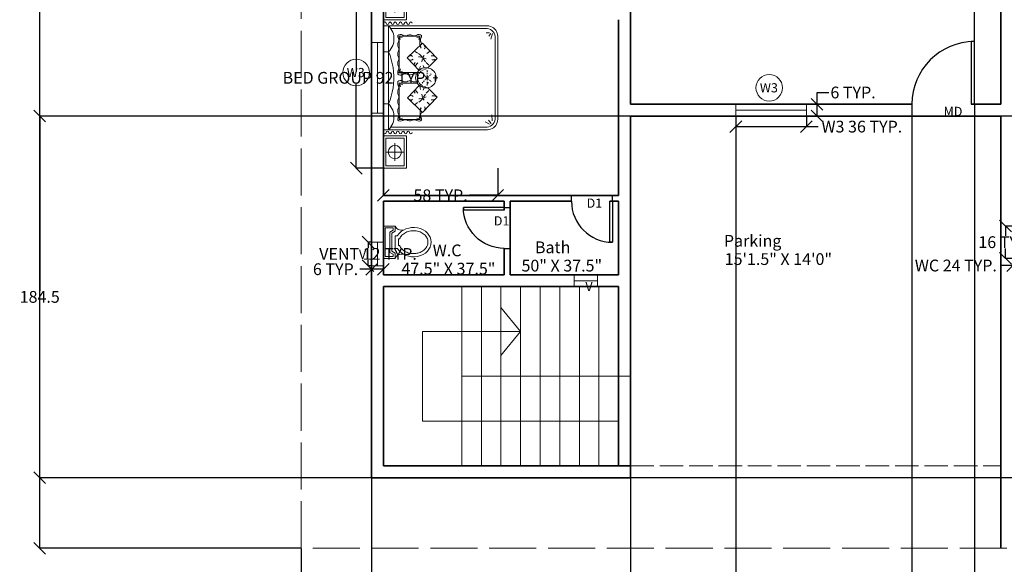
# Model space of a CAD drawing. Units: inches. Extents: x -1198 to -69, y -512 to 437.
# Tile 2 of 50: x -1198 to -696, y -273 to 5. Entities that reach past the tile are written whole.
import ezdxf

# ---------------------------------------------------------------- set-up
doc = ezdxf.new("R2010")
doc.units = ezdxf.units.IN
doc.header["$MEASUREMENT"] = 0
doc.linetypes.add('ACAD_ISO02W100', pattern=[15, 12, -3])
for name, color, linetype, lineweight in [('A-ANNO-DIMS', 2, 'Continuous', 18), ('A-ANNO-SYMB', 7, 'Continuous', 18), ('A-AREA-IDEN', 7, 'Continuous', 18), ('A-FLOR-FIXT', 60, 'Continuous', 18), ('A-FLOR-OPEN', 7, 'ACAD_ISO02W100', 18), ('A-FLOR-STRS', 7, 'Continuous', 18), ('A-FURN', 60, 'Continuous', 18), ('A-WALL', 7, 'Continuous', 35), ('C-PROP', 141, 'ACAD_ISO02W100', 18), ('Doors', 140, 'Continuous', 25), ('ds_furniture_Pen_No__7', 7, 'Continuous', 18), ('windows', 160, 'Continuous', 18)]:
    doc.layers.add(name, color=color, linetype=linetype, lineweight=lineweight)
doc.styles.get("Standard").update_dxf_attribs({"font": 'arial.ttf'})
doc.dimstyles.get("Standard").update_dxf_attribs({"dimtxt": 6, "dimasz": 6, "dimexe": 0.18, "dimexo": 0.0625, "dimgap": 0.09, "dimtad": 0, "dimtih": 1, "dimtoh": 1, "dimdec": 0, "dimzin": 0, "dimdsep": 46, "dimlunit": 4, "dimtxsty": 'Standard', "dimblk": 'OBLIQUE', "dimcen": 0.09, "dimadec": 0, "dimazin": 0, "dimtfac": 1, "dimtdec": 0, "dimtofl": 0, "dimtmove": 0, "dimatfit": 3, "dimfxl": 1, "dimtolj": 1, "dimtzin": 0, "dimarcsym": 0})

# ---------------------------------------------------------------- blocks, each defined once
blk = doc.blocks.new('*U5')
for p, q in [((0, 0), (0, -6)), ((-32, 0), (-32, -6))]:
    blk.add_line(p, q)
blk.add_lwpolyline([(0, 0), (0, 32), (-1.75, 32), (-1.75, 0)], close=True)
blk.add_arc((0, 0), 32, 90, 180)
blk = doc.blocks.new('new')
at = {"layer": 'ds_furniture_Pen_No__7'}
for p, q in [((-1180, 2274), (-1838, 2274)), ((-1838, 2274), (-1838, 1804)), ((-1227, 2227), (-1791, 2227)), ((-1791, 2227), (-1791, 1851)), ((-1509, 2220), (-1509, 1858)), ((-1227, 1851), (-1227, 2227)), ((-1180, 1804), (-1180, 2274)), ((-1058, 159), (-1058, 2274)), ((-1058, 2274), (1058, 2274)), ((-1058, 2274), (1058, 2274)), ((-1058, 159), (-1058, 2274)), ((-529, 2274), (-529, 2169)), ((529, 2274), (529, 2169)), ((1058, 2274), (1058, 159)), ((1058, 2274), (1058, 159)), ((1180, 1804), (1180, 2274)), ((1180, 2274), (1838, 2274)), ((1227, 1851), (1227, 2227)), ((1227, 2227), (1791, 2227)), ((1509, 2220), (1509, 1858)), ((1791, 2227), (1791, 1851)), ((1838, 2274), (1838, 1804)), ((-1690, 2039), (-1328, 2039)), ((1058, 2169), (-1058, 2169)), ((-1058, 2169), (-1028, 2143)), ((-1028, 2143), (-996, 2120)), ((-1005, 165), (-1005, 2124)), ((-996, 2120), (-963, 2101)), ((-963, 2101), (-927, 2084)), ((-927, 2084), (-891, 2071)), ((-891, 2071), (-851, 2063)), ((-851, 2063), (-812, 2059)), ((-812, 2059), (-772, 2059)), ((-772, 2059), (-734, 2063)), ((-734, 2063), (-696, 2071)), ((-696, 2071), (-658, 2084)), ((-658, 2084), (-622, 2101)), ((-622, 2101), (-588, 2120)), ((-588, 2120), (-556, 2143)), ((-556, 2143), (-529, 2169)), ((-529, 2169), (-451, 2139)), ((-451, 2139), (-370, 2114)), ((-370, 2114), (-290, 2092)), ((-290, 2092), (-207, 2075)), ((-207, 2075), (-125, 2065)), ((-125, 2065), (-42, 2061)), ((-42, 2061), (42, 2061)), ((42, 2061), (125, 2065)), ((125, 2065), (207, 2075)), ((207, 2075), (290, 2092)), ((290, 2092), (370, 2114)), ((370, 2114), (451, 2139)), ((451, 2139), (529, 2169)), ((529, 2169), (556, 2143)), ((556, 2143), (588, 2120)), ((588, 2120), (622, 2101)), ((622, 2101), (658, 2084)), ((658, 2084), (696, 2071)), ((696, 2071), (734, 2063)), ((734, 2063), (772, 2059)), ((772, 2059), (812, 2059)), ((812, 2059), (851, 2063)), ((851, 2063), (891, 2071)), ((891, 2071), (927, 2084)), ((927, 2084), (963, 2101)), ((963, 2101), (996, 2120)), ((996, 2120), (1028, 2143)), ((1005, 2124), (1005, 165)), ((1028, 2143), (1058, 2169)), ((1690, 2039), (1328, 2039)), ((-1838, 1804), (-1180, 1804)), ((-1791, 1851), (-1227, 1851)), ((-880, 1932), (-874, 1959)), ((-878, 1904), (-880, 1932)), ((-870, 1879), (-878, 1904)), ((-874, 1959), (-861, 1982)), ((-857, 1855), (-870, 1879)), ((-861, 1982), (-836, 1982)), ((-857, 1798), (-857, 1855)), ((-846, 1528), (-846, 1951)), ((-846, 1951), (-108, 1951)), ((-836, 1982), (-810, 1974)), ((-831, 1930), (-821, 1887)), ((-825, 1944), (-779, 1930)), ((-810, 1974), (-787, 1961)), ((-787, 1961), (-751, 1961)), ((-751, 1961), (-726, 1974)), ((-726, 1974), (-700, 1980)), ((-700, 1980), (-675, 1982)), ((-675, 1982), (-647, 1980)), ((-647, 1980), (-622, 1974)), ((-622, 1974), (-597, 1961)), ((-597, 1961), (-561, 1961)), ((-561, 1961), (-535, 1974)), ((-535, 1974), (-510, 1980)), ((-510, 1980), (-484, 1982)), ((-484, 1982), (-457, 1980)), ((-457, 1980), (-432, 1974)), ((-432, 1974), (-408, 1961)), ((-408, 1961), (-370, 1961)), ((-370, 1961), (-347, 1974)), ((-347, 1974), (-322, 1980)), ((-322, 1980), (-294, 1982)), ((-294, 1982), (-267, 1980)), ((-267, 1980), (-241, 1974)), ((-241, 1974), (-218, 1961)), ((-218, 1961), (-180, 1961)), ((-133, 1940), (-182, 1923)), ((-180, 1961), (-157, 1974)), ((-157, 1974), (-133, 1982)), ((-129, 1923), (-140, 1881)), ((-133, 1982), (-106, 1982)), ((-108, 1951), (-108, 1591)), ((-106, 1982), (-74, 1982)), ((-66, 1879), (-80, 1855)), ((-80, 1855), (-80, 1798)), ((-74, 1982), (-63, 1959)), ((-57, 1904), (-66, 1879)), ((-63, 1959), (-57, 1932)), ((-57, 1932), (-57, 1904)), ((63, 1959), (57, 1932)), ((57, 1932), (57, 1904)), ((57, 1904), (66, 1879)), ((74, 1982), (63, 1959)), ((66, 1879), (80, 1855)), ((106, 1982), (74, 1982)), ((80, 1855), (80, 1798)), ((133, 1982), (106, 1982)), ((844, 1953), (106, 1953)), ((106, 1953), (106, 1593)), ((127, 1925), (138, 1883)), ((131, 1942), (180, 1925)), ((157, 1974), (133, 1982)), ((180, 1961), (157, 1974)), ((218, 1961), (180, 1961)), ((241, 1974), (218, 1961)), ((267, 1980), (241, 1974)), ((294, 1982), (267, 1980)), ((322, 1980), (294, 1982)), ((347, 1974), (322, 1980)), ((370, 1961), (347, 1974)), ((408, 1961), (370, 1961)), ((432, 1974), (408, 1961)), ((457, 1980), (432, 1974)), ((484, 1982), (457, 1980)), ((510, 1980), (484, 1982)), ((535, 1974), (510, 1980)), ((561, 1961), (535, 1974)), ((597, 1961), (561, 1961)), ((622, 1974), (597, 1961)), ((647, 1980), (622, 1974)), ((675, 1982), (647, 1980)), ((700, 1980), (675, 1982)), ((726, 1974), (700, 1980)), ((751, 1961), (726, 1974)), ((787, 1961), (751, 1961)), ((823, 1946), (776, 1932)), ((810, 1974), (787, 1961)), ((836, 1982), (810, 1974)), ((829, 1932), (819, 1889)), ((861, 1982), (836, 1982)), ((844, 1530), (844, 1953)), ((857, 1855), (870, 1879)), ((857, 1798), (857, 1855)), ((874, 1959), (861, 1982)), ((870, 1879), (878, 1904)), ((880, 1932), (874, 1959)), ((878, 1904), (880, 1932)), ((1838, 1804), (1180, 1804)), ((1791, 1851), (1227, 1851)), ((-876, 1748), (-870, 1775)), ((-876, 1722), (-876, 1748)), ((-870, 1695), (-876, 1722)), ((-870, 1775), (-857, 1798)), ((-857, 1671), (-870, 1695)), ((-870, 1602), (-857, 1625)), ((-857, 1625), (-857, 1671)), ((-705, 1475), (-408, 1786)), ((-540, 1627), (-504, 1580)), ((-440, 1743), (-461, 1707)), ((-461, 1707), (-436, 1680)), ((-408, 1786), (-154, 1544)), ((-362, 1697), (-383, 1669)), ((-366, 1750), (-362, 1697)), ((-277, 1648), (-313, 1627)), ((-245, 1627), (-309, 1574)), ((-91, 1595), (-61, 1608)), ((-80, 1798), (-66, 1775)), ((-66, 1695), (-80, 1671)), ((-80, 1671), (-80, 1608)), ((-66, 1775), (-59, 1748)), ((-59, 1722), (-66, 1695)), ((-61, 1608), (-32, 1614)), ((-59, 1748), (-59, 1722)), ((-32, 1614), (0, 1619)), ((0, 1619), (32, 1614)), ((32, 1614), (61, 1608)), ((66, 1775), (59, 1748)), ((59, 1748), (59, 1722)), ((59, 1722), (66, 1695)), ((61, 1608), (91, 1595)), ((80, 1798), (66, 1775)), ((66, 1695), (80, 1671)), ((80, 1671), (80, 1608)), ((406, 1788), (152, 1547)), ((243, 1629), (307, 1576)), ((275, 1650), (311, 1629)), ((364, 1752), (360, 1699)), ((360, 1699), (381, 1671)), ((702, 1477), (406, 1788)), ((459, 1709), (434, 1682)), ((438, 1745), (459, 1709)), ((537, 1629), (501, 1583)), ((870, 1775), (857, 1798)), ((857, 1671), (870, 1695)), ((857, 1625), (857, 1671)), ((870, 1602), (857, 1625)), ((876, 1748), (870, 1775)), ((870, 1695), (876, 1722)), ((876, 1722), (876, 1748)), ((-880, 1549), (-878, 1576)), ((-874, 1521), (-880, 1549)), ((-878, 1576), (-870, 1602)), ((-861, 1498), (-874, 1521)), ((-836, 1498), (-861, 1498)), ((-652, 1528), (-846, 1528)), ((-810, 1506), (-836, 1498)), ((-831, 1549), (-821, 1591)), ((-825, 1534), (-779, 1549)), ((-787, 1519), (-810, 1506)), ((-772, 1517), (-789, 1517)), ((-751, 1519), (-787, 1519)), ((-762, 1517), (-772, 1517)), ((-751, 1517), (-762, 1517)), ((-726, 1506), (-751, 1519)), ((-700, 1500), (-726, 1506)), ((-394, 1178), (-705, 1475)), ((-683, 1498), (-700, 1500)), ((-656, 1517), (-635, 1517)), ((-656, 1439), (-620, 1422)), ((-635, 1517), (-614, 1506)), ((-614, 1506), (-630, 1517)), ((-630, 1517), (-603, 1513)), ((-620, 1422), (-599, 1432)), ((-599, 1432), (-588, 1439)), ((-472, 1523), (-493, 1555)), ((-425, 1481), (-472, 1523)), ((-457, 1443), (-419, 1470)), ((-429, 1538), (-429, 1555)), ((-415, 1481), (-429, 1538)), ((-404, 1443), (-415, 1481)), ((-398, 1475), (-330, 1492)), ((-398, 1439), (-387, 1401)), ((-394, 1460), (-330, 1418)), ((-218, 1449), (-250, 1464)), ((-214, 1528), (-239, 1517)), ((-218, 1449), (-203, 1449)), ((-176, 1528), (-214, 1528)), ((-205, 1418), (-201, 1449)), ((-205, 1386), (-205, 1418)), ((-201, 1449), (-193, 1479)), ((-197, 1401), (-180, 1439)), ((-193, 1479), (-180, 1508)), ((-182, 1555), (-154, 1544)), ((-180, 1508), (-163, 1534)), ((-176, 1528), (-171, 1523)), ((-169, 1479), (-176, 1458)), ((-169, 1479), (-159, 1489)), ((-163, 1534), (-142, 1557)), ((-116, 1538), (-148, 1500)), ((-148, 1528), (-144, 1521)), ((-142, 1557), (-118, 1578)), ((-118, 1578), (-91, 1595)), ((-116, 1538), (-95, 1549)), ((-91, 1468), (-106, 1485)), ((-59, 1443), (-80, 1458)), ((-42, 1574), (-74, 1559)), ((-38, 1428), (-49, 1428)), ((-32, 1580), (-2, 1580)), ((-6, 1396), (-32, 1418)), ((19, 1580), (-11, 1580)), ((-6, 1585), (-6, 1570)), ((-6, 1585), (-6, 1570)), ((4, 1396), (30, 1418)), ((30, 1574), (61, 1559)), ((36, 1428), (47, 1428)), ((57, 1443), (78, 1458)), ((104, 1538), (83, 1549)), ((89, 1468), (104, 1485)), ((91, 1595), (118, 1578)), ((112, 1528), (138, 1502)), ((118, 1578), (142, 1557)), ((142, 1557), (163, 1534)), ((157, 1479), (146, 1489)), ((180, 1557), (152, 1547)), ((157, 1479), (163, 1458)), ((163, 1534), (180, 1508)), ((184, 1401), (167, 1439)), ((173, 1530), (169, 1525)), ((173, 1530), (212, 1530)), ((180, 1508), (193, 1479)), ((193, 1479), (201, 1449)), ((216, 1451), (201, 1451)), ((201, 1449), (205, 1418)), ((205, 1418), (205, 1386)), ((212, 1530), (237, 1519)), ((216, 1451), (248, 1466)), ((258, 1350), (311, 1403)), ((396, 1477), (328, 1494)), ((391, 1462), (328, 1420)), ((396, 1441), (385, 1403)), ((391, 1181), (702, 1477)), ((402, 1445), (413, 1483)), ((413, 1483), (427, 1540)), ((455, 1445), (417, 1473)), ((423, 1483), (470, 1525)), ((427, 1540), (427, 1557)), ((470, 1525), (491, 1557)), ((597, 1434), (586, 1441)), ((618, 1424), (597, 1434)), ((628, 1519), (601, 1515)), ((633, 1519), (611, 1508)), ((611, 1508), (628, 1519)), ((654, 1441), (618, 1424)), ((654, 1519), (633, 1519)), ((650, 1530), (844, 1530)), ((683, 1498), (700, 1500)), ((700, 1500), (726, 1506)), ((726, 1506), (751, 1519)), ((749, 1519), (760, 1519)), ((751, 1519), (787, 1519)), ((760, 1519), (770, 1519)), ((770, 1519), (787, 1519)), ((823, 1536), (776, 1551)), ((787, 1519), (810, 1506)), ((810, 1506), (836, 1498)), ((829, 1551), (819, 1593)), ((836, 1498), (861, 1498)), ((861, 1498), (874, 1521)), ((878, 1576), (870, 1602)), ((874, 1521), (880, 1549)), ((880, 1549), (878, 1576)), ((-540, 1333), (-493, 1386)), ((-451, 1274), (-446, 1301)), ((-451, 1252), (-451, 1274)), ((-436, 1227), (-451, 1252)), ((-394, 1178), (-207, 1369)), ((-383, 1217), (-366, 1238)), ((-366, 1280), (-372, 1280)), ((-366, 1238), (-366, 1280)), ((-260, 1348), (-313, 1401)), ((-199, 1356), (-205, 1386)), ((-188, 1324), (-199, 1356)), ((-176, 1297), (-188, 1324)), ((-157, 1272), (-176, 1297)), ((-123, 1386), (-159, 1386)), ((-133, 1248), (-157, 1272)), ((-110, 1229), (-133, 1248)), ((-80, 1214), (-110, 1229)), ((-80, 1386), (-106, 1386)), ((-74, 1312), (-80, 1301)), ((-51, 1204), (-80, 1214)), ((53, 1221), (-72, 1221)), ((-59, 1386), (-63, 1386)), ((-49, 1333), (-63, 1316)), ((-21, 1197), (-51, 1204)), ((-17, 1375), (-49, 1386)), ((-38, 1343), (-38, 1343)), ((-6, 1369), (-32, 1354)), ((-17, 1386), (-17, 1396)), ((-17, 1396), (-6, 1396)), ((-17, 1375), (-17, 1386)), ((-6, 1369), (-17, 1375)), ((-6, 1396), (-2, 1398)), ((-6, 1369), (-2, 1369)), ((4, 1396), (-2, 1398)), ((4, 1369), (-2, 1369)), ((0, 1164), (0, 1263)), ((15, 1396), (4, 1396)), ((4, 1369), (15, 1375)), ((4, 1369), (30, 1354)), ((15, 1386), (15, 1396)), ((15, 1375), (15, 1386)), ((15, 1375), (47, 1386)), ((51, 1204), (21, 1197)), ((36, 1343), (36, 1343)), ((47, 1333), (61, 1316)), ((80, 1214), (51, 1204)), ((57, 1386), (61, 1386)), ((72, 1312), (78, 1301)), ((78, 1386), (104, 1386)), ((110, 1229), (80, 1214)), ((133, 1248), (110, 1229)), ((121, 1386), (157, 1386)), ((157, 1272), (133, 1248)), ((176, 1297), (157, 1272)), ((188, 1324), (176, 1297)), ((199, 1356), (188, 1324)), ((205, 1386), (199, 1356)), ((391, 1181), (205, 1371)), ((364, 1240), (364, 1282)), ((364, 1282), (370, 1282)), ((381, 1219), (364, 1240)), ((434, 1229), (449, 1255)), ((449, 1276), (444, 1303)), ((449, 1255), (449, 1276)), ((537, 1335), (491, 1388)), ((0, 1197), (-21, 1197)), ((21, 1197), (0, 1197)), ((-941, 116), (-895, 205)), ((-1054, 127), (-1058, 159)), ((-1054, 127), (-1058, 159)), ((-1045, 95), (-1054, 127)), ((-1045, 95), (-1054, 127)), ((-1032, 63), (-1045, 95)), ((-1032, 63), (-1045, 95)), ((-1016, 36), (-1032, 63)), ((-1016, 36), (-1032, 63)), ((-994, 11), (-1016, 36)), ((-994, 11), (-1016, 36)), ((-996, 129), (-1005, 165)), ((-984, 97), (-996, 129)), ((-969, -11), (-994, 11)), ((-969, -11), (-994, 11)), ((-963, 68), (-984, 97)), ((-937, 42), (-963, 68)), ((-908, 21), (-937, 42)), ((-931, 85), (-863, 138)), ((-876, 8), (-908, 21)), ((-840, 0), (-876, 8)), ((-874, 63), (-751, 70)), ((840, 0), (-840, 0)), ((903, 53), (787, 91)), ((876, 8), (840, 0)), ((903, 91), (844, 127)), ((908, 21), (876, 8)), ((937, 42), (908, 21)), ((914, 116), (914, 184)), ((963, 68), (937, 42)), ((984, 97), (963, 68)), ((994, 11), (969, -11)), ((994, 11), (969, -11)), ((996, 129), (984, 97)), ((1016, 36), (994, 11)), ((1016, 36), (994, 11)), ((1005, 165), (996, 129)), ((1032, 63), (1016, 36)), ((1032, 63), (1016, 36)), ((1045, 95), (1032, 63)), ((1045, 95), (1032, 63)), ((1054, 127), (1045, 95)), ((1054, 127), (1045, 95)), ((1058, 159), (1054, 127)), ((1058, 159), (1054, 127)), ((-941, -28), (-969, -11)), ((-941, -28), (-969, -11)), ((-910, -40), (-941, -28)), ((-910, -40), (-941, -28)), ((-878, -49), (-910, -40)), ((-878, -49), (-910, -40)), ((-846, -53), (-878, -49)), ((-846, -53), (-878, -49)), ((846, -53), (-846, -53)), ((846, -53), (-846, -53)), ((878, -49), (846, -53)), ((878, -49), (846, -53)), ((910, -40), (878, -49)), ((910, -40), (878, -49)), ((941, -28), (910, -40)), ((941, -28), (910, -40)), ((969, -11), (941, -28)), ((969, -11), (941, -28))]:
    blk.add_line(p, q, dxfattribs=at)
for centre in [(-1509, 2039), (1509, 2039)]:
    blk.add_circle(centre, 134, dxfattribs=at)
for centre, start, end in [((-1113, 2243), 90, 270), ((-1113, 2191), 270, 90), ((1109, 2191), 90, 270), ((1109, 2243), 270, 90), ((-1113, 2138), 90, 270), ((-1113, 2032), 90, 270), ((-1113, 2085), 270, 90), ((-1113, 2085), 270, 90), ((-1113, 1979), 270, 90), ((1109, 2085), 90, 270), ((1109, 2085), 90, 270), ((1109, 1979), 90, 270), ((1109, 2138), 270, 90), ((1109, 2032), 270, 90), ((-1113, 1926), 90, 270), ((-1113, 1820), 90, 270), ((-1113, 1873), 270, 90), ((1109, 1873), 90, 270), ((1109, 1926), 270, 90), ((1109, 1820), 270, 90), ((-1113, 1715), 90, 270), ((-1113, 1767), 270, 90), ((1109, 1767), 90, 270), ((1109, 1715), 270, 90)]:
    blk.add_arc(centre, 26.4, start, end, dxfattribs=at)
blk = doc.blocks.new('A$C7C8779AE')
for p, q in [((0, 0.74), (0, 0.56)), ((0.5, 0.74), (0, 0.74)), ((0.47, 0.71), (0.03, 0.71)), ((0.03, 0.71), (0.03, 0.59)), ((0.093, 0.64), (0.063, 0.59)), ((0.11, 0.61), (0.08, 0.56)), ((0.093, 0.64), (0.407, 0.64)), ((0.11, 0.61), (0.39, 0.61)), ((0.42, 0.56), (0.39, 0.61)), ((0.437, 0.59), (0.407, 0.64)), ((0.47, 0.59), (0.47, 0.71)), ((0.5, 0.56), (0.5, 0.74)), ((0, 0.56), (0.08, 0.56)), ((0.03, 0.59), (0.063, 0.59)), ((0.15, 0.557), (0.15, 0.52)), ((0.15, 0.557), (0.351, 0.557)), ((0.2, 0.507), (0.2, 0.488)), ((0.2, 0.507), (0.301, 0.507)), ((0.301, 0.507), (0.301, 0.488)), ((0.351, 0.557), (0.351, 0.52)), ((0.42, 0.56), (0.5, 0.56)), ((0.437, 0.59), (0.47, 0.59))]:
    blk.add_line(p, q)
for centre, start, end in [((-0.039, 0.461), 344.642, 68.7339), ((0.539, 0.461), 111.2661, 195.358)]:
    blk.add_arc(centre, 0.106, start, end)
blk.add_ellipse((0.251, 0.274), major_axis=(0, 0.274), ratio=0.828948, start_param=0.459479, end_param=5.823706)
blk.add_open_spline([(0.2, 0.488), (0.17, 0.474), (0.164, 0.47), (0.151, 0.46), (0.144, 0.454), (0.13, 0.439), (0.123, 0.431), (0.111, 0.413), (0.106, 0.404), (0.096, 0.384), (0.091, 0.373), (0.084, 0.352), (0.081, 0.34), (0.076, 0.317), (0.075, 0.305), (0.073, 0.282), (0.073, 0.27), (0.074, 0.246), (0.076, 0.234), (0.08, 0.211), (0.083, 0.2), (0.09, 0.178), (0.095, 0.167), (0.104, 0.147), (0.11, 0.138), (0.122, 0.12), (0.128, 0.112), (0.142, 0.097), (0.149, 0.09), (0.165, 0.078), (0.173, 0.073), (0.189, 0.064), (0.197, 0.06), (0.214, 0.055), (0.222, 0.053), (0.239, 0.05), (0.248, 0.05), (0.266, 0.051), (0.276, 0.052), (0.296, 0.057), (0.306, 0.061), (0.325, 0.071), (0.335, 0.077), (0.353, 0.091), (0.361, 0.099), (0.377, 0.117), (0.384, 0.127), (0.398, 0.149), (0.404, 0.161), (0.414, 0.185), (0.418, 0.198), (0.424, 0.225), (0.426, 0.239), (0.428, 0.267), (0.428, 0.281), (0.426, 0.309), (0.424, 0.323), (0.418, 0.349), (0.414, 0.363), (0.404, 0.387), (0.398, 0.399), (0.385, 0.421), (0.378, 0.431), (0.362, 0.449), (0.353, 0.458), (0.338, 0.469), (0.332, 0.474), (0.301, 0.488)], degree=3, knots=[0.459479, 0.459479, 0.459479, 0.459479, 0.567422, 0.567422, 0.720865, 0.720865, 0.874307, 0.874307, 1.02775, 1.02775, 1.181192, 1.181192, 1.334635, 1.334635, 1.488077, 1.488077, 1.64152, 1.64152, 1.794963, 1.794963, 1.948405, 1.948405, 2.101848, 2.101848, 2.25529, 2.25529, 2.408733, 2.408733, 2.562175, 2.562175, 2.715618, 2.715618, 2.86906, 2.86906, 3.022503, 3.022503, 3.175946, 3.175946, 3.356457, 3.356457, 3.536968, 3.536968, 3.717479, 3.717479, 3.89799, 3.89799, 4.078501, 4.078501, 4.259012, 4.259012, 4.439523, 4.439523, 4.620035, 4.620035, 4.800546, 4.800546, 4.981057, 4.981057, 5.161568, 5.161568, 5.342079, 5.342079, 5.52259, 5.52259, 5.703101, 5.703101, 5.823706, 5.823706, 5.823706, 5.823706])
blk = doc.blocks.new('A')
at = {"xscale": 1000, "yscale": 1000, "zscale": 1000}
blk.add_blockref('A$C7C8779AE', (-251, 0), dxfattribs=at)
blk = doc.blocks.new('WIN-W3-36')
at = {"ltscale": 10}
for p, q in [((0, 6), (0, 0)), ((36, 6), (36, 0)), ((0, 3), (36, 3))]:
    blk.add_line(p, q, dxfattribs=at)
blk = doc.blocks.new('VENT-12')
at = {"ltscale": 10}
for p, q in [((0, 6), (0, 0)), ((12, 6), (12, 0)), ((0, 3), (12, 3))]:
    blk.add_line(p, q, dxfattribs=at)
blk = doc.blocks.new('DOOR-D1-JAMB3')
for p, q in [((0, 0), (0, -3)), ((20.87, 0), (20.87, -3))]:
    blk.add_line(p, q)
blk.add_lwpolyline([(0, 0), (0, 20.87), (1.3, 20.87), (1.3, 0)], close=True)
blk.add_arc((0, 0), 20.87, 0, 90)
blk = doc.blocks.new('STAIR-RETURN')
at = {"ltscale": 10}
for p, q in [((20, 91.5), (20, 0)), ((30, 91.5), (30, 0)), ((40, 91.5), (40, 0)), ((50, 91.5), (50, 0)), ((60, 91.5), (60, 0)), ((70, 91.5), (70, 0)), ((80, 91.5), (80, 0)), ((90, 91.5), (90, 0)), ((50, 68.62), (40, 80.86)), ((0, 22.87), (0, 68.62)), ((0, 68.62), (50, 68.62)), ((50, 68.62), (40, 56.39)), ((20, 45.75), (106, 45.75)), ((100, 22.87), (0, 22.87))]:
    blk.add_line(p, q, dxfattribs=at)
blk = doc.blocks.new('TAG-W3')
at = {"ltscale": 10}
blk.add_circle((0, 0), 6.77, dxfattribs=at)
blk.add_text('W3', height=4.7, dxfattribs=at).set_placement((-4.79, -2.36))
blk = doc.blocks.new('_Oblique')
at = {"color": 0, "linetype": 'ByBlock', "lineweight": -2}
blk.add_line((-0.5, -0.5), (0.5, 0.5), dxfattribs=at)
blk = doc.blocks.new('*D36')
at = {"layer": 'A-ANNO-DIMS', "color": 0, "lineweight": -2, "ltscale": 10, "transparency": 16777216}
for p, q in [((-1018.81, -108.61), (-1020.73, -108.61)), ((-1020.55, -108.61), (-1020.55, -111.51)), ((-1020.55, -120.61), (-1020.55, -117.72)), ((-1018.81, -120.61), (-1020.73, -120.61))]:
    blk.add_line(p, q, dxfattribs=at)
at = {"layer": 'DEFPOINTS', "color": 0, "ltscale": 10, "transparency": 16777216}
for p in [(-1020.55, -108.61), (-1018.75, -108.61), (-1018.75, -120.61)]:
    blk.add_point(p, dxfattribs=at)
at = {"layer": 'A-ANNO-DIMS', "color": 0, "lineweight": -2, "ltscale": 10, "transparency": 16777216, "xscale": 6, "yscale": 6, "zscale": 6}
for p, rotation in [((-1020.55, -108.61), 90), ((-1020.55, -120.61), 270)]:
    blk.add_blockref('_Oblique', p, dxfattribs=dict(at, rotation=rotation))
at = {"layer": 'A-ANNO-DIMS', "color": 0, "ltscale": 10, "transparency": 16777216, "insert": (-1020.55, -114.61), "char_height": 6, "attachment_point": 5}
blk.add_mtext('\\A1;VENT 12 TYP.', dxfattribs=at)
blk = doc.blocks.new('*D37')
at = {"layer": 'A-ANNO-DIMS', "color": 0, "lineweight": -2, "ltscale": 10, "transparency": 16777216}
for p, q in [((-1018.75, -122.41), (-1024.75, -122.41)), ((-1018.75, -120.68), (-1018.75, -122.59)), ((-1012.75, -122.41), (-1018.75, -122.41)), ((-1012.75, -120.68), (-1012.75, -122.59))]:
    blk.add_line(p, q, dxfattribs=at)
at = {"layer": 'DEFPOINTS', "color": 0, "ltscale": 10, "transparency": 16777216}
for p in [(-1018.75, -120.61), (-1018.75, -122.41), (-1012.75, -120.61)]:
    blk.add_point(p, dxfattribs=at)
at = {"layer": 'A-ANNO-DIMS', "color": 0, "lineweight": -2, "ltscale": 10, "transparency": 16777216, "xscale": 6, "yscale": 6, "zscale": 6}
for p, rotation in [((-1018.75, -122.41), 180.0000000000012), ((-1012.75, -122.41), 1.199e-12)]:
    blk.add_blockref('_Oblique', p, dxfattribs=dict(at, rotation=rotation))
at = {"layer": 'A-ANNO-DIMS', "color": 0, "ltscale": 10, "transparency": 16777216, "insert": (-1037.13, -122.41), "char_height": 6, "attachment_point": 5}
blk.add_mtext('\\A1;6 TYP.', dxfattribs=at)
blk = doc.blocks.new('*D38')
at = {"layer": 'A-ANNO-DIMS', "color": 0, "lineweight": -2, "ltscale": 10, "transparency": 16777216}
for p, q in [((-1012.81, 21.34), (-1026.76, 21.34)), ((-1026.58, 21.34), (-1026.58, -21.58)), ((-1026.58, -70.88), (-1026.58, -27.97)), ((-1012.81, -70.88), (-1026.76, -70.88))]:
    blk.add_line(p, q, dxfattribs=at)
at = {"layer": 'DEFPOINTS', "color": 0, "ltscale": 10, "transparency": 16777216}
for p in [(-1026.58, 21.34), (-1012.75, 21.34), (-1012.75, -70.88)]:
    blk.add_point(p, dxfattribs=at)
at = {"layer": 'A-ANNO-DIMS', "color": 0, "lineweight": -2, "ltscale": 10, "transparency": 16777216, "xscale": 6, "yscale": 6, "zscale": 6}
for p, rotation in [((-1026.58, 21.34), 90), ((-1026.58, -70.88), 270)]:
    blk.add_blockref('_Oblique', p, dxfattribs=dict(at, rotation=rotation))
at = {"layer": 'A-ANNO-DIMS', "color": 0, "ltscale": 10, "transparency": 16777216, "insert": (-1026.58, -24.77), "char_height": 6, "attachment_point": 5}
blk.add_mtext('\\A1;BED GROUP 92 TYP.', dxfattribs=at)
blk = doc.blocks.new('*D39')
at = {"layer": 'A-ANNO-DIMS', "color": 0, "lineweight": -2, "ltscale": 10, "transparency": 16777216}
for p, q in [((-1012.75, -70.94), (-1012.75, -84.89)), ((-954.38, -70.94), (-954.38, -84.89)), ((-1012.75, -84.71), (-998.26, -84.71)), ((-954.38, -84.71), (-968.87, -84.71))]:
    blk.add_line(p, q, dxfattribs=at)
at = {"layer": 'DEFPOINTS', "color": 0, "ltscale": 10, "transparency": 16777216}
for p in [(-1012.75, -70.88), (-954.38, -70.88), (-1012.75, -84.71)]:
    blk.add_point(p, dxfattribs=at)
at = {"layer": 'A-ANNO-DIMS', "color": 0, "lineweight": -2, "ltscale": 10, "transparency": 16777216, "xscale": 6, "yscale": 6, "zscale": 6, "rotation": 180}
blk.add_blockref('_Oblique', (-1012.75, -84.71), dxfattribs=at)
at = {"layer": 'A-ANNO-DIMS', "color": 0, "lineweight": -2, "ltscale": 10, "transparency": 16777216, "xscale": 6, "yscale": 6, "zscale": 6}
blk.add_blockref('_Oblique', (-954.38, -84.71), dxfattribs=at)
at = {"layer": 'A-ANNO-DIMS', "color": 0, "ltscale": 10, "transparency": 16777216, "insert": (-983.56, -84.71), "char_height": 6, "attachment_point": 5}
blk.add_mtext('\\A1;58 TYP.', dxfattribs=at)
blk = doc.blocks.new('*D44')
at = {"layer": 'A-ANNO-DIMS', "color": 0, "lineweight": -2, "ltscale": 10, "transparency": 16777216}
for p, q in [((-691.75, -120.52), (-697.75, -120.52)), ((-691.75, -116.92), (-691.75, -120.7)), ((-667.34, -120.52), (-691.75, -120.52)), ((-667.34, -116.92), (-667.34, -120.7))]:
    blk.add_line(p, q, dxfattribs=at)
at = {"layer": 'DEFPOINTS', "color": 0, "ltscale": 10, "transparency": 16777216}
for p in [(-691.75, -116.86), (-691.75, -120.52), (-667.34, -116.86)]:
    blk.add_point(p, dxfattribs=at)
at = {"layer": 'A-ANNO-DIMS', "color": 0, "lineweight": -2, "ltscale": 10, "transparency": 16777216, "xscale": 6, "yscale": 6, "zscale": 6, "rotation": 180}
blk.add_blockref('_Oblique', (-691.75, -120.52), dxfattribs=at)
at = {"layer": 'A-ANNO-DIMS', "color": 0, "lineweight": -2, "ltscale": 10, "transparency": 16777216, "xscale": 6, "yscale": 6, "zscale": 6}
blk.add_blockref('_Oblique', (-667.34, -120.52), dxfattribs=at)
at = {"layer": 'A-ANNO-DIMS', "color": 0, "ltscale": 10, "transparency": 16777216, "insert": (-720.71, -120.52), "char_height": 6, "attachment_point": 5}
blk.add_mtext('\\A1;WC 24 TYP.', dxfattribs=at)
blk = doc.blocks.new('*D45')
at = {"layer": 'A-ANNO-DIMS', "color": 0, "lineweight": -2, "ltscale": 10, "transparency": 16777216}
for p, q in [((-691.81, -100.37), (-695.59, -100.37)), ((-695.41, -100.37), (-695.41, -105.46)), ((-695.41, -116.86), (-695.41, -111.77)), ((-691.81, -116.86), (-695.59, -116.86))]:
    blk.add_line(p, q, dxfattribs=at)
at = {"layer": 'DEFPOINTS', "color": 0, "ltscale": 10, "transparency": 16777216}
for p in [(-695.41, -100.37), (-691.75, -100.37), (-691.75, -116.86)]:
    blk.add_point(p, dxfattribs=at)
at = {"layer": 'A-ANNO-DIMS', "color": 0, "lineweight": -2, "ltscale": 10, "transparency": 16777216, "xscale": 6, "yscale": 6, "zscale": 6}
for p, rotation in [((-695.41, -100.37), 90), ((-695.41, -116.86), 270)]:
    blk.add_blockref('_Oblique', p, dxfattribs=dict(at, rotation=rotation))
at = {"layer": 'A-ANNO-DIMS', "color": 0, "ltscale": 10, "transparency": 16777216, "insert": (-695.41, -108.61), "char_height": 6, "attachment_point": 5}
blk.add_mtext('\\A1;16 TYP.', dxfattribs=at)
blk = doc.blocks.new('*D46')
at = {"layer": 'A-ANNO-DIMS', "color": 0, "lineweight": -2, "ltscale": 10, "transparency": 16777216}
for p, q in [((-832.94, -44.33), (-832.94, -49.85)), ((-796.94, -44.33), (-796.94, -49.85)), ((-832.94, -49.67), (-796.94, -49.67)), ((-796.94, -49.67), (-790.94, -49.67))]:
    blk.add_line(p, q, dxfattribs=at)
at = {"layer": 'DEFPOINTS', "color": 0, "ltscale": 10, "transparency": 16777216}
for p in [(-832.94, -44.27), (-796.94, -44.27), (-796.94, -49.67)]:
    blk.add_point(p, dxfattribs=at)
at = {"layer": 'A-ANNO-DIMS', "color": 0, "lineweight": -2, "ltscale": 10, "transparency": 16777216, "xscale": 6, "yscale": 6, "zscale": 6, "rotation": 180}
blk.add_blockref('_Oblique', (-832.94, -49.67), dxfattribs=at)
at = {"layer": 'A-ANNO-DIMS', "color": 0, "lineweight": -2, "ltscale": 10, "transparency": 16777216, "xscale": 6, "yscale": 6, "zscale": 6}
blk.add_blockref('_Oblique', (-796.94, -49.67), dxfattribs=at)
at = {"layer": 'A-ANNO-DIMS', "color": 0, "ltscale": 10, "transparency": 16777216, "insert": (-768.67, -49.67), "char_height": 6, "attachment_point": 5}
blk.add_mtext('\\A1;W3 36 TYP.', dxfattribs=at)
blk = doc.blocks.new('*D47')
at = {"layer": 'A-ANNO-DIMS', "color": 0, "lineweight": -2, "ltscale": 10, "transparency": 16777216}
for p, q in [((-791.54, -38.27), (-791.54, -32.27)), ((-791.54, -32.27), (-785.54, -32.27)), ((-796.88, -38.27), (-791.36, -38.27)), ((-791.54, -44.27), (-791.54, -38.27)), ((-796.88, -44.27), (-791.36, -44.27))]:
    blk.add_line(p, q, dxfattribs=at)
at = {"layer": 'DEFPOINTS', "color": 0, "ltscale": 10, "transparency": 16777216}
for p in [(-796.94, -38.27), (-791.54, -38.27), (-796.94, -44.27)]:
    blk.add_point(p, dxfattribs=at)
at = {"layer": 'A-ANNO-DIMS', "color": 0, "lineweight": -2, "ltscale": 10, "transparency": 16777216, "xscale": 6, "yscale": 6, "zscale": 6}
for p, rotation in [((-791.54, -38.27), 90), ((-791.54, -44.27), 270)]:
    blk.add_blockref('_Oblique', p, dxfattribs=dict(at, rotation=rotation))
at = {"layer": 'A-ANNO-DIMS', "color": 0, "ltscale": 10, "transparency": 16777216, "insert": (-773.16, -32.27), "char_height": 6, "attachment_point": 5}
blk.add_mtext('\\A1;6 TYP.', dxfattribs=at)
blk = doc.blocks.new('*D60')
at = {"layer": 'A-ANNO-DIMS', "color": 0, "lineweight": -2, "ltscale": 10, "transparency": 16777216}
for p, q in [((-1054.75, -264.83), (-1054.75, -507.84)), ((-334.75, -264.83), (-334.75, -507.84)), ((-1054.75, -507.66), (-701.43, -507.66)), ((-334.75, -507.66), (-688.07, -507.66))]:
    blk.add_line(p, q, dxfattribs=at)
at = {"layer": 'DEFPOINTS', "color": 0, "ltscale": 10, "transparency": 16777216}
for p in [(-1054.75, -264.77), (-334.75, -264.77), (-334.75, -507.66)]:
    blk.add_point(p, dxfattribs=at)
at = {"layer": 'A-ANNO-DIMS', "color": 0, "lineweight": -2, "ltscale": 10, "transparency": 16777216, "xscale": 6, "yscale": 6, "zscale": 6, "rotation": 180}
blk.add_blockref('_Oblique', (-1054.75, -507.66), dxfattribs=at)
at = {"layer": 'A-ANNO-DIMS', "color": 0, "lineweight": -2, "ltscale": 10, "transparency": 16777216, "xscale": 6, "yscale": 6, "zscale": 6}
blk.add_blockref('_Oblique', (-334.75, -507.66), dxfattribs=at)
at = {"layer": 'A-ANNO-DIMS', "color": 0, "ltscale": 10, "transparency": 16777216, "insert": (-694.75, -507.66), "char_height": 6, "attachment_point": 5}
blk.add_mtext('\\A1;720', dxfattribs=at)
blk = doc.blocks.new('*D61')
at = {"layer": 'A-ANNO-DIMS', "color": 0, "lineweight": -2, "ltscale": 10, "transparency": 16777216}
for p, q in [((-1054.81, 299.23), (-1188.2, 299.23)), ((-1188.02, 299.23), (-1188.02, 20.38)), ((-1188.02, -264.77), (-1188.02, 14.07)), ((-1054.81, -264.77), (-1188.2, -264.77))]:
    blk.add_line(p, q, dxfattribs=at)
at = {"layer": 'DEFPOINTS', "color": 0, "ltscale": 10, "transparency": 16777216}
for p in [(-1054.75, 299.23), (-1188.02, -264.77), (-1054.75, -264.77)]:
    blk.add_point(p, dxfattribs=at)
at = {"layer": 'A-ANNO-DIMS', "color": 0, "lineweight": -2, "ltscale": 10, "transparency": 16777216, "xscale": 6, "yscale": 6, "zscale": 6}
for p, rotation in [((-1188.02, 299.23), 90), ((-1188.02, -264.77), 270)]:
    blk.add_blockref('_Oblique', p, dxfattribs=dict(at, rotation=rotation))
at = {"layer": 'A-ANNO-DIMS', "color": 0, "ltscale": 10, "transparency": 16777216, "insert": (-1188.02, 17.23), "char_height": 6, "attachment_point": 5}
blk.add_mtext('\\A1;564', dxfattribs=at)
blk = doc.blocks.new('*D62')
at = {"layer": 'A-ANNO-DIMS', "color": 0, "lineweight": -2, "ltscale": 10, "transparency": 16777216}
for p, q in [((-1018.75, -228.83), (-1018.75, -507.84)), ((-370.75, -228.83), (-370.75, -507.84)), ((-1018.75, -507.66), (-701.49, -507.66)), ((-370.75, -507.66), (-688.01, -507.66))]:
    blk.add_line(p, q, dxfattribs=at)
at = {"layer": 'DEFPOINTS', "color": 0, "ltscale": 10, "transparency": 16777216}
for p in [(-1018.75, -228.77), (-370.75, -228.77), (-370.75, -507.66)]:
    blk.add_point(p, dxfattribs=at)
at = {"layer": 'A-ANNO-DIMS', "color": 0, "lineweight": -2, "ltscale": 10, "transparency": 16777216, "xscale": 6, "yscale": 6, "zscale": 6, "rotation": 180}
blk.add_blockref('_Oblique', (-1018.75, -507.66), dxfattribs=at)
at = {"layer": 'A-ANNO-DIMS', "color": 0, "lineweight": -2, "ltscale": 10, "transparency": 16777216, "xscale": 6, "yscale": 6, "zscale": 6}
blk.add_blockref('_Oblique', (-370.75, -507.66), dxfattribs=at)
at = {"layer": 'A-ANNO-DIMS', "color": 0, "ltscale": 10, "transparency": 16777216, "insert": (-694.75, -507.66), "char_height": 6, "attachment_point": 5}
blk.add_mtext('\\A1;648', dxfattribs=at)
blk = doc.blocks.new('*D72')
at = {"layer": 'A-ANNO-DIMS', "color": 0, "lineweight": -2, "ltscale": 10, "transparency": 16777216}
for p, q in [((-743.13, -44.33), (-743.13, -507.84)), ((-711.13, -44.33), (-711.13, -507.84)), ((-743.13, -507.66), (-731.49, -507.66)), ((-711.13, -507.66), (-722.78, -507.66))]:
    blk.add_line(p, q, dxfattribs=at)
at = {"layer": 'DEFPOINTS', "color": 0, "ltscale": 10, "transparency": 16777216}
for p in [(-743.13, -44.27), (-711.13, -44.27), (-711.13, -507.66)]:
    blk.add_point(p, dxfattribs=at)
at = {"layer": 'A-ANNO-DIMS', "color": 0, "lineweight": -2, "ltscale": 10, "transparency": 16777216, "xscale": 6, "yscale": 6, "zscale": 6, "rotation": 180}
blk.add_blockref('_Oblique', (-743.13, -507.66), dxfattribs=at)
at = {"layer": 'A-ANNO-DIMS', "color": 0, "lineweight": -2, "ltscale": 10, "transparency": 16777216, "xscale": 6, "yscale": 6, "zscale": 6}
blk.add_blockref('_Oblique', (-711.13, -507.66), dxfattribs=at)
at = {"layer": 'A-ANNO-DIMS', "color": 0, "ltscale": 10, "transparency": 16777216, "insert": (-727.13, -507.66), "char_height": 6, "attachment_point": 5}
blk.add_mtext('\\A1;32', dxfattribs=at)
blk = doc.blocks.new('*D75')
at = {"layer": 'A-ANNO-DIMS', "color": 0, "lineweight": -2, "ltscale": 10, "transparency": 16777216}
for p, q in [((-376.81, -44.27), (-1188.2, -44.27)), ((-1188.02, -44.27), (-1188.02, -133.37)), ((-1188.02, -228.77), (-1188.02, -139.68)), ((-370.81, -228.77), (-1188.2, -228.77))]:
    blk.add_line(p, q, dxfattribs=at)
at = {"layer": 'DEFPOINTS', "color": 0, "ltscale": 10, "transparency": 16777216}
for p in [(-1188.02, -44.27), (-376.75, -44.27), (-370.75, -228.77)]:
    blk.add_point(p, dxfattribs=at)
at = {"layer": 'A-ANNO-DIMS', "color": 0, "lineweight": -2, "ltscale": 10, "transparency": 16777216, "xscale": 6, "yscale": 6, "zscale": 6}
for p, rotation in [((-1188.02, -44.27), 90), ((-1188.02, -228.77), 270)]:
    blk.add_blockref('_Oblique', p, dxfattribs=dict(at, rotation=rotation))
at = {"layer": 'A-ANNO-DIMS', "color": 0, "ltscale": 10, "transparency": 16777216, "insert": (-1188.02, -136.52), "char_height": 6, "attachment_point": 5}
blk.add_mtext('\\A1;184.5', dxfattribs=at)
blk = doc.blocks.new('*D76')
at = {"layer": 'A-ANNO-DIMS', "color": 0, "lineweight": -2, "ltscale": 10, "transparency": 16777216}
for p, q in [((-711.13, -38.21), (-711.13, 433.18)), ((-711.13, 433), (-697.75, 433)), ((-697.75, -38.21), (-697.75, 433.18)), ((-697.75, 433), (-691.75, 433))]:
    blk.add_line(p, q, dxfattribs=at)
at = {"layer": 'DEFPOINTS', "color": 0, "ltscale": 10, "transparency": 16777216}
for p in [(-697.75, 433), (-711.13, -38.27), (-697.75, -38.27)]:
    blk.add_point(p, dxfattribs=at)
at = {"layer": 'A-ANNO-DIMS', "color": 0, "lineweight": -2, "ltscale": 10, "transparency": 16777216, "xscale": 6, "yscale": 6, "zscale": 6, "rotation": 180}
blk.add_blockref('_Oblique', (-711.13, 433), dxfattribs=at)
at = {"layer": 'A-ANNO-DIMS', "color": 0, "lineweight": -2, "ltscale": 10, "transparency": 16777216, "xscale": 6, "yscale": 6, "zscale": 6}
blk.add_blockref('_Oblique', (-697.75, 433), dxfattribs=at)
at = {"layer": 'A-ANNO-DIMS', "color": 0, "ltscale": 10, "transparency": 16777216, "insert": (-681.81, 433), "char_height": 6, "attachment_point": 5}
blk.add_mtext('\\A1;13.38', dxfattribs=at)
blk = doc.blocks.new('*D77')
at = {"layer": 'A-ANNO-DIMS', "color": 0, "lineweight": -2, "ltscale": 10, "transparency": 16777216}
for p, q in [((-886.75, -44.33), (-886.75, -507.84)), ((-832.94, -44.33), (-832.94, -507.84)), ((-886.75, -507.66), (-869.48, -507.66)), ((-832.94, -507.66), (-850.21, -507.66))]:
    blk.add_line(p, q, dxfattribs=at)
at = {"layer": 'DEFPOINTS', "color": 0, "ltscale": 10, "transparency": 16777216}
for p in [(-886.75, -44.27), (-832.94, -44.27), (-832.94, -507.66)]:
    blk.add_point(p, dxfattribs=at)
at = {"layer": 'A-ANNO-DIMS', "color": 0, "lineweight": -2, "ltscale": 10, "transparency": 16777216, "xscale": 6, "yscale": 6, "zscale": 6, "rotation": 180}
blk.add_blockref('_Oblique', (-886.75, -507.66), dxfattribs=at)
at = {"layer": 'A-ANNO-DIMS', "color": 0, "lineweight": -2, "ltscale": 10, "transparency": 16777216, "xscale": 6, "yscale": 6, "zscale": 6}
blk.add_blockref('_Oblique', (-832.94, -507.66), dxfattribs=at)
at = {"layer": 'A-ANNO-DIMS', "color": 0, "ltscale": 10, "transparency": 16777216, "insert": (-859.85, -507.66), "char_height": 6, "attachment_point": 5}
blk.add_mtext('\\A1;53.81', dxfattribs=at)

msp = doc.modelspace()

# ---------------------------------------------------------------- linework, layer by layer
at = {"layer": 'A-FLOR-OPEN'}
for p, q in [((-886.7509, -222.7723), (-697.7509, -222.7723)), ((-886.7509, -228.7723), (-697.7509, -228.7723))]:
    msp.add_line(p, q, dxfattribs=at)
at = {"layer": 'A-WALL', "ltscale": 10}
for p, q in [((-1018.7509, 263.2277), (-1018.7509, -228.7723)), ((-1012.7509, 35.2277), (-1012.7509, -84.7723)), ((-886.7509, 35.2277), (-886.7509, -38.2723)), ((-697.7509, 35.2277), (-697.7509, -38.2723)), ((-892.7509, 4.874), (-892.7509, -84.7723)), ((-743.1319, -38.2723), (-886.7509, -38.2723)), ((-697.7509, -38.2723), (-712.8819, -38.2723)), ((-697.7509, -44.2723), (-886.7509, -44.2723)), ((-886.7509, -44.2723), (-886.7509, -125.2723)), ((-697.7509, -44.2723), (-697.7509, -125.2723)), ((-892.7509, -84.7723), (-1012.7509, -84.7723)), ((-1012.7509, -87.7723), (-1012.7509, -125.2723)), ((-962.2509, -87.7723), (-1012.7509, -87.7723)), ((-951.0669, -87.7723), (-962.2509, -87.7723)), ((-951.0669, -87.7723), (-951.0669, -92.2048)), ((-948.0669, -87.7723), (-948.0669, -125.2723)), ((-916.782, -87.7723), (-948.0669, -87.7723)), ((-892.7509, -87.7723), (-897.2167, -87.7723)), ((-892.7509, -87.7723), (-892.7509, -125.2723)), ((-886.7509, -87.7723), (-886.7509, -131.2723)), ((-697.7509, -87.7723), (-697.7509, -131.2723)), ((-951.0669, -111.7701), (-951.0669, -125.2723)), ((-962.2509, -125.2723), (-1012.7509, -125.2723)), ((-951.0669, -125.2723), (-962.2509, -125.2723)), ((-892.7509, -125.2723), (-948.0669, -125.2723)), ((-892.7509, -131.2723), (-1012.7509, -131.2723)), ((-1012.7509, -131.2723), (-1012.7509, -222.7723)), ((-892.7509, -131.2723), (-892.7509, -222.7723)), ((-886.7509, -131.2723), (-886.7509, -228.7723)), ((-697.7509, -131.2723), (-697.7509, -228.7723)), ((-1012.7509, -222.7723), (-886.7509, -222.7723)), ((-1018.7509, -228.7723), (-886.7509, -228.7723)), ((-697.7509, -228.7723), (-697.7509, -264.7723))]:
    msp.add_line(p, q, dxfattribs=at)
at = {"layer": 'C-PROP', "ltscale": 2}
msp.add_lwpolyline([(-1054.7509, 299.2277), (-334.7509, 299.2277), (-334.7509, -264.7723), (-1054.7509, -264.7723)], close=True, dxfattribs=at)

# ---------------------------------------------------------------- block references
at = {"layer": 'A-ANNO-SYMB'}
for p in [(-1026.6373, -22.0827), (-815.8941, -29.8595)]:
    msp.add_blockref('TAG-W3', p, dxfattribs=at)
at = {"layer": 'A-FLOR-FIXT', "ltscale": 10, "xscale": 0.0329718540314781, "yscale": 0.0329718540314781, "zscale": 0.0329718540314781, "rotation": 89.99999999999999}
msp.add_blockref('A', (-988.3364, -108.5941), dxfattribs=at)
at = {"layer": 'A-FLOR-STRS'}
msp.add_blockref('STAIR-RETURN', (-992.751, -222.772), dxfattribs=at)
at = {"layer": 'A-FURN', "xscale": 0.0250833463801972, "yscale": 0.0250833463801972, "zscale": 0.0250833463801972, "rotation": 90}
msp.add_blockref('new', (-955.702, -24.7723), dxfattribs=at)
at = {"layer": 'Doors'}
msp.add_blockref('*U5', (-711.1319, -38.2723), dxfattribs=at)
at = {"layer": 'Doors', "rotation": 180}
msp.add_blockref('DOOR-D1-JAMB3', (-895.9123, -87.7723), dxfattribs=at)
at = {"layer": 'Doors', "extrusion": (0, 0, -1), "zscale": -1, "rotation": 269.9999999999994}
msp.add_blockref('DOOR-D1-JAMB3', (951.0669, -90.9004), dxfattribs=at)
at = {"layer": 'windows'}
for name, p, rotation in [('WIN-W3-36', (-1012.7512, -42.772), 89.99999999999967), ('VENT-12', (-1012.7512, -120.6129), 90.00000000000115), ('VENT-12', (-903.4789, -125.2727), 180)]:
    msp.add_blockref(name, p, dxfattribs=dict(at, rotation=rotation))
msp.add_blockref('WIN-W3-36', (-832.941, -44.272), dxfattribs=at)

# ---------------------------------------------------------------- texts
at = {"layer": 'A-ANNO-SYMB', "ltscale": 10}
for s, height, p in [('MD', 4.69957, (-726.9671, -44.2723)), ('D1', 4.69957, (-909.0676, -91.05)), ('D1', 4.69957, (-956.4254, -100.0945)), ('V', 4.6996, (-1025.1905, -117.1805)), ('V', 4.6996, (-909.6937, -133.6031))]:
    msp.add_text(s, height=height, dxfattribs=at).set_placement(p)
at = {"layer": 'A-AREA-IDEN', "ltscale": 10, "char_height": 6, "attachment_point": 1}
for s, insert in [('Parking', (-839.0415, -104.9183)), ('W.C', (-987.5723, -109.8143)), ('Bath', (-935.407, -108.2495)), ('15\'1.5" X 14\'0"', (-838.6221, -114.2454)), ('47.5" X 37.5"', (-1003.5231, -119.1414)), ('50" X 37.5"', (-942.2707, -117.5766))]:
    msp.add_mtext_dynamic_manual_height_columns(s, width=57.976527, gutter_width=30, heights=[0], dxfattribs=dict(at, insert=insert))

# ---------------------------------------------------------------- dimensions: what is measured, and where the dimension line sits
at = {"layer": 'A-ANNO-DIMS', "ltscale": 10}
for base, p1, p2, override, picture, middle in [((-697.7509, 433.0036), (-711.1319, -38.2723), (-697.7509, -38.2723), {"dimdec": 2, "dimlfac": 1, "dimrnd": 0, "dimzin": 0, "dimdsep": 46, "dimlunit": 2}, '*D76', (-681.8137, 433.0036)), ((-832.9414, -507.6552), (-886.7509, -44.2723), (-832.9414, -44.2723), {"dimdec": 2, "dimlfac": 1, "dimrnd": 0, "dimzin": 0, "dimdsep": 46, "dimlunit": 2}, '*D77', (-859.8461, -507.6552)), ((-711.1319, -507.6552), (-743.1319, -44.2723), (-711.1319, -44.2723), {"dimdec": 0, "dimlfac": 1, "dimrnd": 0, "dimzin": 0, "dimdsep": 46, "dimlunit": 2}, '*D72', (-727.1319, -507.6552)), ((-370.7509, -507.6552), (-1018.7509, -228.7723), (-370.7509, -228.7723), {"dimdec": 0, "dimlfac": 1, "dimrnd": 0, "dimzin": 0, "dimdsep": 46, "dimlunit": 2}, '*D62', (-694.7509, -507.6552)), ((-334.7509, -507.6552), (-1054.7509, -264.7723), (-334.7509, -264.7723), {"dimdec": 0, "dimlfac": 1, "dimrnd": 0, "dimzin": 0, "dimdsep": 46, "dimlunit": 2}, '*D60', (-694.7509, -507.6552))]:
    dim = msp.add_linear_dim(base=base, p1=p1, p2=p2, dimstyle='Standard', override=override, dxfattribs=at)
    dim.commit()
    dim.dimension.update_dxf_attribs({"geometry": picture, "text_midpoint": middle})
for base, p1, p2, override, picture, middle in [((-1188.0248, -264.7723), (-1054.7509, 299.2277), (-1054.7509, -264.7723), {"dimdec": 0, "dimlfac": 1, "dimrnd": 0, "dimzin": 0, "dimdsep": 46, "dimlunit": 2}, '*D61', (-1188.0248, 17.2277)), ((-1188.0248, -44.2723), (-370.7509, -228.7723), (-376.7509, -44.2723), {"dimdec": 1, "dimlfac": 1, "dimrnd": 0, "dimzin": 0, "dimdsep": 46, "dimlunit": 2}, '*D75', (-1188.0248, -136.5223))]:
    dim = msp.add_linear_dim(base=base, p1=p1, p2=p2, angle=90, dimstyle='Standard', override=override, dxfattribs=at)
    dim.commit()
    dim.dimension.update_dxf_attribs({"geometry": picture, "text_midpoint": middle})
for base, p1, p2, angle, text, picture, middle in [((-1026.5835, 21.3366), (-1012.7509, -70.8813), (-1012.7509, 21.3366), 90, 'BED GROUP <> TYP.', '*D38', (-1026.5835, -24.7723)), ((-791.5414, -38.2723), (-796.9414, -44.2723), (-796.9414, -38.2723), 90, '<> TYP.', '*D47', (-773.1628, -32.2723)), ((-1012.7509, -84.714), (-954.3753, -70.8813), (-1012.7509, -70.8813), 180, '<> TYP.', '*D39', (-983.5631, -84.714)), ((-695.413, -100.3697), (-691.7509, -116.8556), (-691.7509, -100.3697), 90, '<> TYP.', '*D45', (-695.413, -108.6126)), ((-1020.5509, -108.6126), (-1018.7509, -120.6126), (-1018.7509, -108.6126), 90, 'VENT <> TYP.', '*D36', (-1020.5509, -114.6126)), ((-691.7509, -120.5177), (-667.3364, -116.8556), (-691.7509, -116.8556), 180, 'WC <> TYP.', '*D44', (-720.7133, -120.5177)), ((-1018.7509, -122.4126), (-1012.7509, -120.6126), (-1018.7509, -120.6126), 180, '<> TYP.', '*D37', (-1037.1294, -122.4126))]:
    dim = msp.add_linear_dim(base=base, p1=p1, p2=p2, angle=angle, text=text, dimstyle='Standard', override={"dimdec": 0, "dimlfac": 1, "dimrnd": 0, "dimzin": 0, "dimdsep": 46, "dimlunit": 2}, dxfattribs=at)
    dim.commit()
    dim.dimension.update_dxf_attribs({"geometry": picture, "text_midpoint": middle})
dim = msp.add_linear_dim(base=(-796.9414, -49.6723), p1=(-832.9414, -44.2723), p2=(-796.9414, -44.2723), text='W3 <> TYP.', dimstyle='Standard', override={"dimdec": 0, "dimlfac": 1, "dimrnd": 0, "dimzin": 0, "dimdsep": 46, "dimlunit": 2}, dxfattribs=at)
dim.commit()
dim.dimension.update_dxf_attribs({"geometry": '*D46', "text_midpoint": (-768.6747, -49.6723)})

doc.saveas('drawing.dxf')
